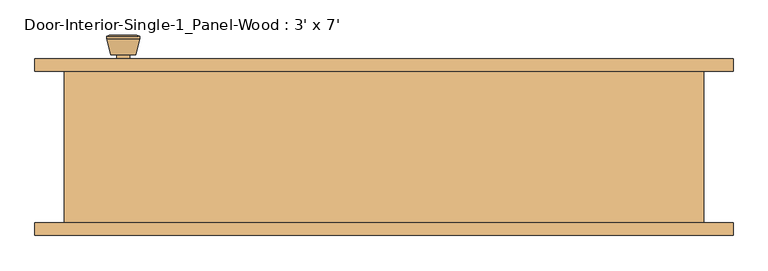
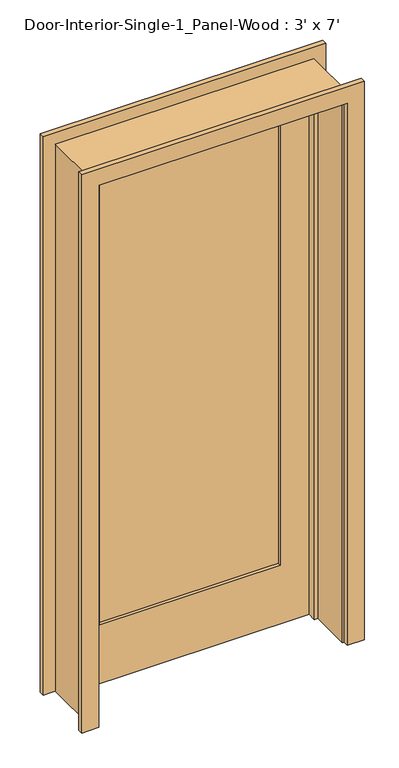
"""IFC4 building model written with IfcOpenShell, lengths in millimetres: door geometry, Door-Interior-Single-1_Panel-Wood : 3' x 7'."""

from ifc_helpers import new_model, si_unit, point, frame, frame_2d, origin, place, context, project, spatial, polyline, circle_curve, trimmed, segment, composite_curve, outline, extrude, faceted_brep, source, transform, mapped, element, save
from ifc_brep_helpers import plane_surface, cylinder_surface, revolved_surface, advanced_brep


def door_interior_single_1_panel_wood_3_x_7_3b97b8e7(model_context):
    return source(origin(), model_context, "Body", "SolidModel", [
        advanced_brep(
        [(-393.7, 70.2, 914.4), (-383.7, 70.2, 914.4), (-403.7, 70.2, 914.4), (-373.2241324, 21.2, 914.4), (-393.7, 21.2, 914.4), (-414.1758676, 21.2, 914.4), (-368.7, 23.0278681, 914.4), (-418.7, 23.0278681, 914.4), (-368.7, 26.4915463, 914.4), (-418.7, 26.4915463, 914.4), (-375.063764, 51.2, 914.4), (-412.336236, 51.2, 914.4), (-383.7, 51.2, 914.4), (-403.7, 51.2, 914.4)],
        [
            (0, 1),
            (1, 2, circle_curve(frame((-393.7, 70.2, 914.4), z_axis=(0.0, 1.0, 0.0), x_axis=(-1.0, 0.0, 0.0)), 10.0)),
            (2, 0),
            (2, 1, circle_curve(frame((-393.7, 70.2, 914.4), z_axis=(0.0, 1.0, 0.0), x_axis=(-1.0, 0.0, 0.0)), 10.0)),
            (3, 4),
            (4, 5),
            (5, 3, circle_curve(frame((-393.7, 21.2, 914.4), z_axis=(0.0, -1.0, 0.0), x_axis=(-1.0, 0.0, 0.0)), 20.4758676)),
            (3, 5, circle_curve(frame((-393.7, 21.2, 914.4), z_axis=(0.0, -1.0, 0.0), x_axis=(-1.0, 0.0, 0.0)), 20.4758676)),
            (6, 3),
            (5, 7),
            (7, 6, circle_curve(frame((-393.7, 23.0278681, 914.4), z_axis=(0.0, -1.0, 0.0), x_axis=(-1.0, 0.0, 0.0)), 25.0)),
            (6, 7, circle_curve(frame((-393.7, 23.0278681, 914.4), z_axis=(0.0, -1.0, 0.0), x_axis=(-1.0, 0.0, 0.0)), 25.0)),
            (8, 6),
            (7, 9),
            (9, 8, circle_curve(frame((-393.7, 26.4915463, 914.4), z_axis=(0.0, -1.0, 0.0), x_axis=(-1.0, 0.0, 0.0)), 25.0)),
            (8, 9, circle_curve(frame((-393.7, 26.4915463, 914.4), z_axis=(0.0, -1.0, 0.0), x_axis=(-1.0, 0.0, 0.0)), 25.0)),
            (10, 8),
            (9, 11),
            (11, 10, circle_curve(frame((-393.7, 51.2, 914.4), z_axis=(0.0, -1.0, 0.0), x_axis=(-1.0, 0.0, 0.0)), 18.636236)),
            (10, 11, circle_curve(frame((-393.7, 51.2, 914.4), z_axis=(0.0, -1.0, 0.0), x_axis=(-1.0, 0.0, 0.0)), 18.636236)),
            (12, 10),
            (11, 13),
            (13, 12, circle_curve(frame((-393.7, 51.2, 914.4), z_axis=(0.0, -1.0, 0.0), x_axis=(-1.0, 0.0, 0.0)), 10.0)),
            (12, 13, circle_curve(frame((-393.7, 51.2, 914.4), z_axis=(0.0, -1.0, 0.0), x_axis=(-1.0, 0.0, 0.0)), 10.0)),
            (1, 12),
            (13, 2),
        ],
        [
            plane_surface(frame((-393.7, 70.2, 914.4), z_axis=(0.0, 1.0, 0.0), x_axis=(-1.0, 0.0, 0.0))),
            plane_surface(frame((-393.7, 21.2, 914.4), z_axis=(0.0, -1.0, 0.0), x_axis=(-1.0, 0.0, 0.0))),
            revolved_surface(polyline([(-414.1758676, 21.2, 914.4), (-418.7, 23.0278681, 914.4)]), (-393.7, 70.2, 914.4), (0.0, 1.0, 0.0)),
            cylinder_surface(frame((-393.7, 70.2, 914.4), z_axis=(0.0, 1.0, 0.0), x_axis=(-1.0, 0.0, 0.0)), 25.0),
            revolved_surface(polyline([(-418.7, 26.4915463, 914.4), (-412.336236, 51.2, 914.4)]), (-393.7, 70.2, 914.4), (0.0, 1.0, 0.0)),
            plane_surface(frame((-393.7, 51.2, 914.4), z_axis=(0.0, 1.0, 0.0), x_axis=(-1.0, 0.0, 0.0))),
            cylinder_surface(frame((-393.7, 70.2, 914.4), z_axis=(0.0, 1.0, 0.0), x_axis=(-1.0, 0.0, 0.0)), 10.0),
        ],
        [
            (0, [[1, 2, 3]]),
            (0, [[-3, 4, -1]]),
            (1, [[5, 6, 7]]),
            (1, [[-6, -5, 8]]),
            (2, [[9, -7, 10, 11]]),
            (2, [[-10, -8, -9, 12]]),
            (3, [[13, -11, 14, 15]]),
            (3, [[-14, -12, -13, 16]]),
            (4, [[17, -15, 18, 19]]),
            (4, [[-18, -16, -17, 20]]),
            (5, [[21, -19, 22, 23]]),
            (5, [[-22, -20, -21, 24]]),
            (6, [[25, -23, 26, -2]]),
            (6, [[-26, -24, -25, -4]]),
        ],
    ),
        extrude(outline(composite_curve([segment(trimmed(circle_curve(frame_2d((914.4, -393.7)), 30.0), [point((914.4, -423.7))], [point((914.4, -363.7))], False, "CARTESIAN"), True, "CONTINUOUS"), segment(trimmed(circle_curve(frame_2d((914.4, -393.7)), 30.0), [point((914.4, -363.7))], [point((914.4, -423.7))], False, "CARTESIAN"), True, "CONTINUOUS")], self_intersect=False)), frame((0.0, 70.2, 0.0), z_axis=(0.0, 1.0, 0.0), x_axis=(0.0, 0.0, 1.0)), (0.0, 0.0, 1.0), 6.0),
        advanced_brep(
        [(-393.7, 117.125, 914.4), (-403.7, 117.125, 914.4), (-383.7, 117.125, 914.4), (-373.2241324, 166.125, 914.4), (-414.1758676, 166.125, 914.4), (-393.7, 166.125, 914.4), (-368.7, 164.2971319, 914.4), (-418.7, 164.2971319, 914.4), (-368.7, 160.8334537, 914.4), (-418.7, 160.8334537, 914.4), (-375.063764, 136.125, 914.4), (-412.336236, 136.125, 914.4), (-383.7, 136.125, 914.4), (-403.7, 136.125, 914.4)],
        [
            (0, 1),
            (1, 2, circle_curve(frame((-393.7, 117.125, 914.4), z_axis=(0.0, -1.0, 0.0), x_axis=(-1.0, 0.0, 0.0)), 10.0)),
            (2, 0),
            (2, 1, circle_curve(frame((-393.7, 117.125, 914.4), z_axis=(0.0, -1.0, 0.0), x_axis=(-1.0, 0.0, 0.0)), 10.0)),
            (3, 4, circle_curve(frame((-393.7, 166.125, 914.4), z_axis=(0.0, 1.0, 0.0), x_axis=(-1.0, 0.0, 0.0)), 20.4758676)),
            (4, 5),
            (5, 3),
            (4, 3, circle_curve(frame((-393.7, 166.125, 914.4), z_axis=(0.0, 1.0, 0.0), x_axis=(-1.0, 0.0, 0.0)), 20.4758676)),
            (6, 7, circle_curve(frame((-393.7, 164.2971319, 914.4), z_axis=(0.0, 1.0, 0.0), x_axis=(-1.0, 0.0, 0.0)), 25.0)),
            (7, 4),
            (3, 6),
            (7, 6, circle_curve(frame((-393.7, 164.2971319, 914.4), z_axis=(0.0, 1.0, 0.0), x_axis=(-1.0, 0.0, 0.0)), 25.0)),
            (8, 9, circle_curve(frame((-393.7, 160.8334537, 914.4), z_axis=(0.0, 1.0, 0.0), x_axis=(-1.0, 0.0, 0.0)), 25.0)),
            (9, 7),
            (6, 8),
            (9, 8, circle_curve(frame((-393.7, 160.8334537, 914.4), z_axis=(0.0, 1.0, 0.0), x_axis=(-1.0, 0.0, 0.0)), 25.0)),
            (10, 11, circle_curve(frame((-393.7, 136.125, 914.4), z_axis=(0.0, 1.0, 0.0), x_axis=(-1.0, 0.0, 0.0)), 18.636236)),
            (11, 9),
            (8, 10),
            (11, 10, circle_curve(frame((-393.7, 136.125, 914.4), z_axis=(0.0, 1.0, 0.0), x_axis=(-1.0, 0.0, 0.0)), 18.636236)),
            (12, 13, circle_curve(frame((-393.7, 136.125, 914.4), z_axis=(0.0, 1.0, 0.0), x_axis=(-1.0, 0.0, 0.0)), 10.0)),
            (13, 11),
            (10, 12),
            (13, 12, circle_curve(frame((-393.7, 136.125, 914.4), z_axis=(0.0, 1.0, 0.0), x_axis=(-1.0, 0.0, 0.0)), 10.0)),
            (1, 13),
            (12, 2),
        ],
        [
            plane_surface(frame((-393.7, 117.125, 914.4), z_axis=(0.0, -1.0, 0.0), x_axis=(-1.0, 0.0, 0.0))),
            plane_surface(frame((-393.7, 166.125, 914.4), z_axis=(0.0, 1.0, 0.0), x_axis=(-1.0, 0.0, 0.0))),
            revolved_surface(polyline([(-414.1758676, 166.125, 914.4), (-418.7, 164.2971319, 914.4)]), (-393.7, 117.125, 914.4), (0.0, -1.0, 0.0)),
            cylinder_surface(frame((-393.7, 117.125, 914.4), z_axis=(0.0, -1.0, 0.0), x_axis=(-1.0, 0.0, 0.0)), 25.0),
            revolved_surface(polyline([(-418.7, 160.8334537, 914.4), (-412.336236, 136.125, 914.4)]), (-393.7, 117.125, 914.4), (0.0, -1.0, 0.0)),
            plane_surface(frame((-393.7, 136.125, 914.4), z_axis=(0.0, -1.0, 0.0), x_axis=(-1.0, 0.0, 0.0))),
            cylinder_surface(frame((-393.7, 117.125, 914.4), z_axis=(0.0, -1.0, 0.0), x_axis=(-1.0, 0.0, 0.0)), 10.0),
        ],
        [
            (0, [[1, 2, 3]]),
            (0, [[-3, 4, -1]]),
            (1, [[5, 6, 7]]),
            (1, [[8, -7, -6]]),
            (2, [[9, 10, -5, 11]]),
            (2, [[12, -11, -8, -10]]),
            (3, [[13, 14, -9, 15]]),
            (3, [[16, -15, -12, -14]]),
            (4, [[17, 18, -13, 19]]),
            (4, [[20, -19, -16, -18]]),
            (5, [[21, 22, -17, 23]]),
            (5, [[24, -23, -20, -22]]),
            (6, [[-2, 25, -21, 26]]),
            (6, [[-4, -26, -24, -25]]),
        ],
    ),
        extrude(outline(composite_curve([segment(trimmed(circle_curve(frame_2d((914.4, -393.7)), 30.0), [point((914.4, -423.7))], [point((914.4, -363.7))], False, "CARTESIAN"), True, "CONTINUOUS"), segment(trimmed(circle_curve(frame_2d((914.4, -393.7)), 30.0), [point((914.4, -363.7))], [point((914.4, -423.7))], False, "CARTESIAN"), True, "CONTINUOUS")], self_intersect=False)), frame((0.0, 111.125, 0.0), z_axis=(0.0, 1.0, 0.0), x_axis=(0.0, 0.0, 1.0)), (0.0, 0.0, 1.0), 6.0),
        faceted_brep([(482.6, 111.125, 0.0), (482.6, -117.475, 0.0), (457.2, -117.475, 0.0), (457.2, 41.275, 0.0), (444.5, 41.275, 0.0), (444.5, 76.2, 0.0), (457.2, 76.2, 0.0), (457.2, 111.125, 0.0), (482.6, 111.125, 2159.0), (482.6, -117.475, 2159.0), (-482.6, -117.475, 2159.0), (-482.6, -117.475, 0.0), (-457.2, -117.475, 0.0), (-457.2, -117.475, 2133.6), (457.2, -117.475, 2133.6), (457.2, 41.275, 2133.6), (-457.2, 41.275, 2133.6), (-457.2, 41.275, 0.0), (-444.5, 41.275, 0.0), (-444.5, 41.275, 2120.9), (444.5, 41.275, 2120.9), (444.5, 76.2, 2120.9), (-444.5, 76.2, 2120.9), (-444.5, 76.2, 0.0), (-457.2, 76.2, 0.0), (-457.2, 76.2, 2133.6), (457.2, 76.2, 2133.6), (457.2, 111.125, 2133.6), (-457.2, 111.125, 2133.6), (-457.2, 111.125, 0.0), (-482.6, 111.125, 0.0), (-482.6, 111.125, 2159.0)], [[[0, 1, 2, 3, 4, 5, 6, 7]], [[1, 0, 8, 9]], [[2, 1, 9, 10, 11, 12, 13, 14]], [[3, 2, 14, 15]], [[4, 3, 15, 16, 17, 18, 19, 20]], [[5, 4, 20, 21]], [[6, 5, 21, 22, 23, 24, 25, 26]], [[7, 6, 26, 27]], [[0, 7, 27, 28, 29, 30, 31, 8]], [[9, 8, 31, 10]], [[15, 14, 13, 16]], [[21, 20, 19, 22]], [[27, 26, 25, 28]], [[30, 29, 24, 23, 18, 17, 12, 11]], [[10, 31, 30, 11]], [[16, 13, 12, 17]], [[22, 19, 18, 23]], [[28, 25, 24, 29]]]),
        extrude(outline(polyline([(2133.6, -457.2), (0.0, -457.2), (0.0, 457.2), (2133.6, 457.2), (2133.6, -457.2)]), holes=[polyline([(2014.5375, -336.55), (2014.5375, 336.55), (231.775, 336.55), (231.775, -336.55), (2014.5375, -336.55)])]), frame((0.0, 76.2, 0.0), z_axis=(0.0, 1.0, 0.0), x_axis=(0.0, 0.0, 1.0)), (0.0, 0.0, 1.0), 34.925),
        extrude(outline(polyline([(336.55, 87.8416667), (-336.55, 87.8416667), (-336.55, 99.4833333), (336.55, 99.4833333), (336.55, 87.8416667)])), frame((0.0, 0.0, 231.775), z_axis=(0.0, 0.0, 1.0), x_axis=(1.0, 0.0, 0.0)), (0.0, 0.0, 1.0), 1782.7625),
        extrude(outline(polyline([(0.0, 463.55), (0.0, 527.05), (2203.45, 527.05), (2203.45, -527.05), (0.0, -527.05), (0.0, -463.55), (2139.95, -463.55), (2139.95, 463.55), (0.0, 463.55)])), frame((0.0, 111.125, 0.0), z_axis=(0.0, 1.0, 0.0), x_axis=(0.0, 0.0, 1.0)), (0.0, 0.0, 1.0), 19.05),
        extrude(outline(polyline([(0.0, 463.55), (0.0, 527.05), (2203.45, 527.05), (2203.45, -527.05), (0.0, -527.05), (0.0, -463.55), (2139.95, -463.55), (2139.95, 463.55), (0.0, 463.55)])), frame((0.0, -136.525, 0.0), z_axis=(0.0, 1.0, 0.0), x_axis=(0.0, 0.0, 1.0)), (0.0, 0.0, 1.0), 19.05),
    ])


if __name__ == "__main__":
    model = new_model("IFC4")
    model_context = context("Model", 3, world=origin())
    ifc_project = project(units=[si_unit("LENGTHUNIT", "METRE", prefix="MILLI")], contexts=[model_context])
    site = spatial("IfcSite", under=ifc_project)
    building = spatial("IfcBuilding", under=site)
    placement = place(None, origin())
    door_interior_single_1_panel_wood_3_x_7_shape = door_interior_single_1_panel_wood_3_x_7_3b97b8e7(model_context)
    element("IfcDoor", 1, ObjectType="Door-Interior-Single-1_Panel-Wood : 3' x 7'", at=placement, inside=building, context=model_context, shape_type="MappedRepresentation", body=[
        mapped(door_interior_single_1_panel_wood_3_x_7_shape, transform((0.0, 0.0, 0.0), x_axis=(1.0, 0.0, 0.0), y_axis=(0.0, 1.0, 0.0), z_axis=(0.0, 0.0, 1.0))),
    ])
    save(model, "model.ifc")

# Revit data of these elements
# Type "Door-Interior-Single-1_Panel-Wood : 3' x 7'"
#   Type Mark = "10"
#   Assembly Code = "C1020300"
#   Analytic Construction = "Wooden"
#   Top Rail = 0' - 4 11/16"
#   Thickness = 0' - 1 3/8"
#   Thermal Resistance (R) = 2.5876 (h·ft²·°F)/BTU
#   Swing Angle [instance default] = 90.00°
#   Stiles = 0' - 4 3/4"
#   Rough Width = 3' - 2"
#   Rough Height = 7' - 1"
#   Height = 7' - 0"
#   Width = 3' - 0"
#   Heat Transfer Coefficient (U) = 0.3865 BTU/(h·ft²·°F)
#   Bottom Rail = 0' - 9 1/8"
#   Trim Material = DOOR 3'6" X 7'
#   Panel Material = DOOR 3'6" X 7'
#   Frame Material = DOOR 3'6" X 7'
#   Door Handle Material = Aluminum
#   Visual Light Transmittance = 0
#   Solar Heat Gain Coefficient = 0
#   Wall Closure = (empty or 0)
#   Function = (empty or 0)
# Element 1 (IfcDoor, "Door-Interior-Single-1_Panel-Wood : 3' x 7'")
#   Materials on its faces: "DOOR 3'6\" X 7'", "Aluminum"
# Materials
#   "DOOR 3'6\" X 7'": class "Generic", colour RGB 120 120 120, transparency 0, Cost = 0
#   "Aluminum": class "Metal", colour RGB 247 247 247, transparency 0, Description = "Aluminum 6061", Cost = 0
